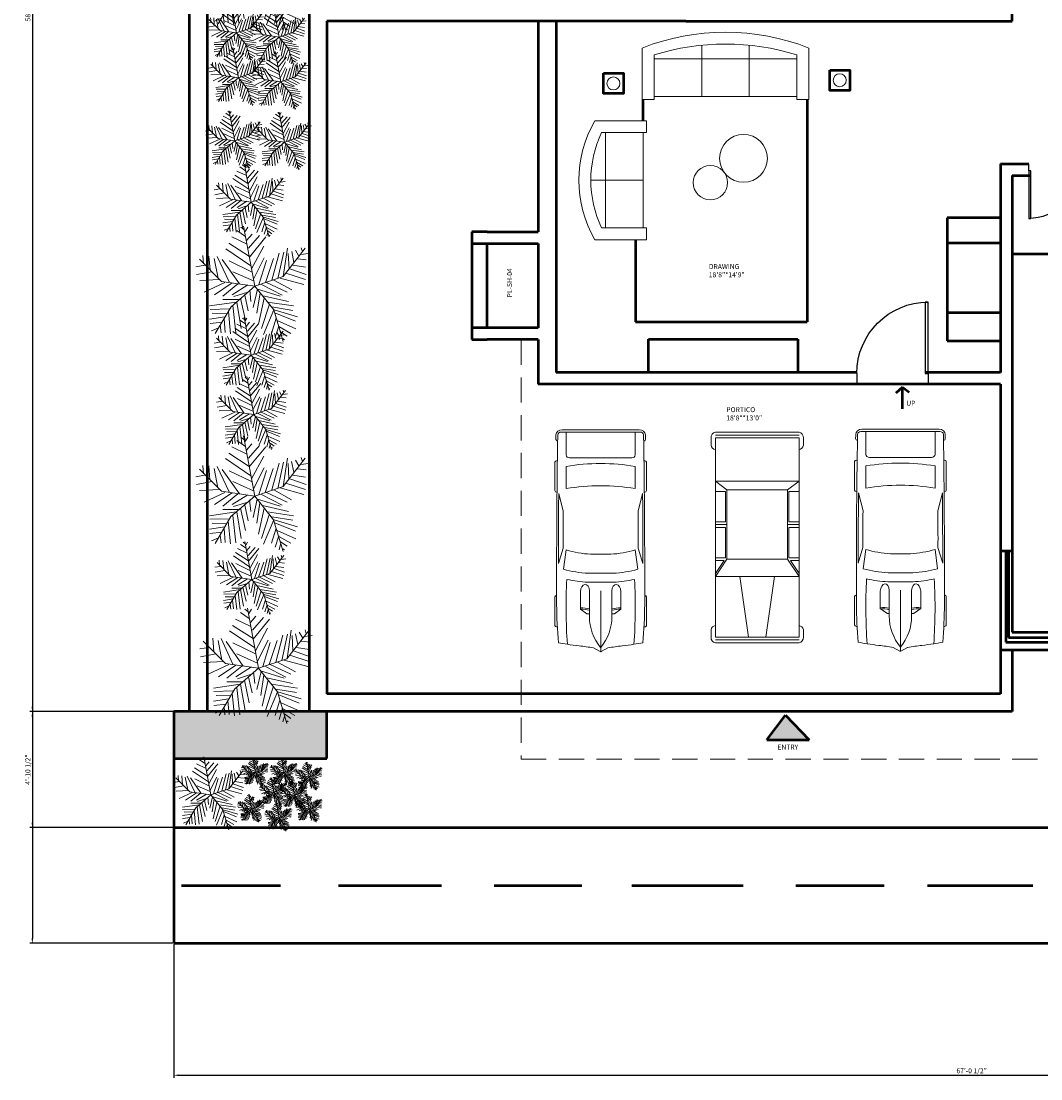
# Model space of a CAD drawing. Units: inches. Extents: x 5312 to 23584, y 2846 to 7447.
# Tile 1 of 12: x 8876 to 9390, y 2846 to 3379. Entities that reach past the tile are written whole.
import ezdxf

# ---------------------------------------------------------------- set-up
doc = ezdxf.new("R2010")
doc.units = ezdxf.units.IN
doc.linetypes.add('DASHED', pattern=[19.05, 12.7, -6.35])
for name, color, linetype, lineweight in [('A-ANNO-DIMS', 2, 'Continuous', 18), ('A-ANNO-TEXT', 3, 'Continuous', 18), ('A-AREA-IDEN', 7, 'Continuous', 18), ('A-DOOR', 4, 'Continuous', 25), ('A-EQPM-VEHI', 8, 'Continuous', 18), ('A-FLOR-OVHD', 8, 'DASHED', 18), ('A-FLOR-PATT', 252, 'Continuous', 13), ('A-FURN', 8, 'Continuous', 18), ('A-WALL', 7, 'Continuous', 50), ('L-PLNT', 82, 'Continuous', 13)]:
    doc.layers.add(name, color=color, linetype=linetype, lineweight=lineweight)
doc.styles.get("Standard").update_dxf_attribs({"font": 'arial.ttf'})
doc.dimstyles.new('ISO-25', dxfattribs={"dimtxt": 2.5, "dimasz": 2.5, "dimexe": 1.25, "dimexo": 0.625, "dimtad": 1, "dimlunit": 3, "dimtxsty": 'Standard', "dimcen": 2.5, "dimadec": 0, "dimazin": 0, "dimtfac": 1, "dimtmove": 0, "dimatfit": 3, "dimfxl": 1, "dimarcsym": 0})

# ---------------------------------------------------------------- blocks, each defined once
blk = doc.blocks.new('Sofa - Roundback 7 ft.')
for p, q in [((-12.00002, -32.4421), (-12.00003, -6.5971)), ((11.99997, -32.4421), (11.99998, -6.5971)), ((-36.000027, -34), (-36.000027, -11.4696)), ((-35.999844, -13.3819), (35.9998, -13.3819)), ((35.99998, -34), (35.99998, -11.4696)), ((-36.000027, -32.4421), (35.99998, -32.4421))]:
    blk.add_line(p, q)
for points in [[(-36.000027, -34), (-42.000027, -34), (-42.000027, -8)], [(41.99998, -8), (41.99998, -34), (35.99998, -34)]]:
    blk.add_lwpolyline(points)
for centre, radius, start, end in [((0, -114.25), 114.25, 68.43141, 111.5686), ((-0.00001, -127.1968), 121.1968, 72.72033, 107.2797)]:
    blk.add_arc(centre, radius, start, end)
blk = doc.blocks.new('Sofa - Roundback Loveseat 5 ft.')
for p, q in [((0, -32.44198), (0, -5.99998)), ((-24, -33.99998), (-24, -11.46958)), ((-23.9998, -13.38178), (23.99986, -13.38178)), ((24.00004, -33.99998), (24.00004, -11.46958)), ((-24, -32.44198), (24.00004, -32.44198))]:
    blk.add_line(p, q)
for points in [[(-24, -33.99998), (-30, -33.99998), (-30, -7.99998)], [(30.00004, -7.99998), (30.00004, -33.99998), (24.00004, -33.99998)]]:
    blk.add_lwpolyline(points)
for centre, radius, start, end in [((0, -60.24998), 60.24998, 60.13715, 119.8628), ((0, -61.38438), 55.38444, 64.32083, 115.6792)]:
    blk.add_arc(centre, radius, start, end)
blk = doc.blocks.new('*U14')
for p, q in [((21.1, 37.41), (21.1, 36.83)), ((46.55, 38.89), (22.35, 38.89)), ((47.8, 37.39), (47.8, 37.41)), ((87.99, 31.87), (74.76, 35.92)), ((135.45, 37.07), (135.45, 37.41)), ((136.7, 38.89), (160.9, 38.89)), ((162.15, 37.41), (162.15, 36.77)), ((70.03, 31.54), (86.41, 29.35)), ((134.31, 35.6), (119.29, 31.78)), ((138.42, 29.35), (157.25, 29.35)), ((186.47, 29.35), (167.01, 29.35)), ((186.47, -33.5), (186.47, 33.5)), ((188.4, -32.76), (188.4, 32.76)), ((164.52, 26.39), (164.52, -26.39)), ((29.77, 9.51), (51.68, 9.51)), ((32.12, 9.51), (32.12, 11.15)), ((32.27, 11.63), (36.13, 17.17)), ((36.13, 17.17), (50.94, 17.17)), ((58.92, -10.77), (58.92, 10.77)), ((66.55, -10.53), (66.55, 10.53)), ((186.47, -10.53), (186.47, 10.53)), ((3.27, 6.13), (0.1, 0.41)), ((82.74, 8.5), (82.74, -8.5)), ((0, 0), (51.68, 0)), ((0.1, -0.41), (3.27, -6.13)), ((29.77, -9.51), (51.68, -9.51)), ((32.12, -9.51), (32.12, -11.15)), ((32.27, -11.63), (36.13, -17.17)), ((36.13, -17.17), (50.94, -17.17)), ((86.41, -29.35), (70.03, -31.54)), ((87.99, -31.87), (74.76, -35.92)), ((134.31, -35.6), (119.29, -31.78)), ((157.25, -29.35), (138.42, -29.35)), ((167.01, -29.35), (186.47, -29.35)), ((21.1, -37.41), (21.1, -36.83)), ((46.55, -38.89), (22.35, -38.89)), ((47.8, -37.39), (47.8, -37.41)), ((135.45, -37.07), (135.45, -37.41)), ((136.7, -38.89), (160.9, -38.89)), ((162.15, -37.41), (162.15, -36.77))]:
    blk.add_line(p, q)
for centre, major_axis, ratio, start_param, end_param in [((41.19, -490.86), (0, 528.23), 0.842304, 0.00281, 0.075598), ((22.35, 37.41), (0, -1.48), 0.842304, 3.141593, 4.712389), ((64.48, -10555.62), (0, 10593.03), 0.842304, -0.013397, 0.002797), ((46.55, 37.41), (0, 1.48), 0.842304, -1.570796, 0), ((64.48, -10555.62), (0, -10591.55), 0.842304, 3.133765, 3.140441), ((136.7, 37.41), (0, -1.48), 0.842304, 3.141593, 4.712389), ((160.9, 37.41), (0, 1.48), 0.842304, -1.570796, 0), ((180.63, 35.84), (0, 2.22), 0.842304, -0.013017, 1.249894), ((64.48, -10556.36), (0, 10595.31), 0.842304, -0.013397, -0.013017), ((183.98, 33.5), (0, -2.96), 0.842304, 1.570796, 3.128196), ((183.98, 32.76), (0, -5.25), 0.842304, 1.570796, 3.128196), ((259.18, -27.52), (0, -305.3), 0.842304, 4.528606, 4.561838), ((266.03, -27.52), (0, 313.31), 0.842304, 1.367076, 1.39176), ((37.47, -593.96), (0, -623.33), 0.842304, 3.096046, 3.200911), ((134.4, 5.39), (0, -89.78), 0.842304, 4.449482, 4.652344), ((135.29, 5.39), (0, 81.77), 0.842304, 1.245306, 1.50788), ((149.6, 2.8), (0, -79.58), 0.842304, 4.372215, 4.640744), ((95.79, -3666.35), (0, -3698.24), 0.842304, 3.134049, 3.144098), ((17.08, 0), (0, 147.02), 0.842304, 4.511394, 4.913384), ((35.91, 0), (0, 147.02), 0.842304, 4.511394, 4.913384), ((167.01, 26.39), (0, 2.96), 0.842304, 0, 1.570796), ((-204.49, 52.4), (0, -250.96), 0.842304, 1.385369, 1.434372), ((29.77, -46.66), (0, 56.17), 0.842304, 0, 0.590319), ((32.75, 11.15), (0, 0.74), 0.842304, 0.879714, 1.570796), ((13.04, 17.01), (0, 27.42), 0.842304, 4.435146, 4.718221), ((14.2, 17.01), (0, 27.42), 0.842304, 4.435146, 4.718221), ((50.79, 13.34), (6.34, -0.36), 0.603834, -1.395552, 1.581315), ((0.62, 0), (0, -0.74), 0.842304, 4.131459, 5.293319), ((-204.49, -52.4), (0, 250.96), 0.842304, -1.434372, -1.385369), ((29.77, 46.66), (0, 56.17), 0.842304, 2.551274, 3.141593), ((149.6, -2.8), (0, -79.58), 0.842304, -1.499151, -1.230623), ((32.75, -11.15), (0, -0.74), 0.842304, 4.712389, 5.403472), ((13.04, -17.01), (0, -27.42), 0.842304, 1.564964, 1.848039), ((14.2, -17.01), (0, -27.42), 0.842304, 1.564964, 1.848039), ((134.4, -5.39), (0, -89.78), 0.842304, -1.510751, -1.307889), ((135.29, -5.39), (0, -81.77), 0.842304, -1.50788, -1.245306), ((259.18, 27.52), (0, 305.3), 0.842304, 1.721348, 1.754579), ((167.01, -26.39), (0, -2.96), 0.842304, 4.712389, 6.283185), ((266.03, 27.52), (0, 313.31), 0.842304, 1.749832, 1.774517), ((37.47, 593.96), (0, -623.33), 0.842304, -0.059319, 0.045547), ((41.19, 490.86), (0, -528.23), 0.842304, -0.075598, -0.00281), ((64.48, 10555.62), (0, -10591.55), 0.842304, 0.001152, 0.007828), ((95.79, 3666.35), (0, -3698.24), 0.842304, -0.002505, 0.007544), ((183.98, -33.5), (0, 2.96), 0.842304, 3.15499, 4.712389), ((183.98, -32.76), (0, -5.25), 0.842304, 0.013397, 1.570796), ((22.35, -37.41), (0, 1.48), 0.842304, 1.570796, 3.141593), ((64.48, 10555.62), (0, 10593.03), 0.842304, 3.138796, 3.15499), ((46.55, -37.41), (0, -1.48), 0.842304, 0, 1.570796), ((136.7, -37.41), (0, -1.48), 0.842304, -1.570796, 0), ((160.9, -37.41), (0, 1.48), 0.842304, 3.141593, 4.712389), ((180.63, -35.84), (0, -2.22), 0.842304, -1.249894, 0.013017), ((64.48, 10556.36), (0, 10595.31), 0.842304, 3.15461, 3.15499)]:
    blk.add_ellipse(centre, major_axis=major_axis, ratio=ratio, start_param=start_param, end_param=end_param)
at = {"extrusion": (0, 0, -1)}
blk.add_ellipse((50.79, -13.34), major_axis=(6.34, 0.36), ratio=0.603834, start_param=-1.395552, end_param=1.581315, dxfattribs=at)
blk = doc.blocks.new('*U15')
for p, q in [((5.44, 42.31), (12.12, 42.31)), ((189.69, 42.31), (183.01, 42.31)), ((0.1, -0.41), (0.1, 38.35)), ((2.77, -0.41), (2.77, 38.31)), ((5.44, -0.41), (5.44, 38.24)), ((5.45, 38.31), (16.12, 38.31)), ((16.12, 38.31), (180.34, 38.31)), ((61.52, -0.41), (61.52, 38.31)), ((61.52, 38.31), (77.54, 27.62)), ((64.19, 38.31), (76.2, 30.29)), ((76.2, 30.29), (76.2, 38.31)), ((78.87, 38.31), (78.87, 28.96)), ((106.91, 28.96), (106.91, 38.31)), ((109.58, 27.62), (109.58, 38.31)), ((112.25, 38.31), (112.25, 28.96)), ((140.29, 28.96), (140.29, 38.31)), ((141.62, 27.62), (149.64, 38.31)), ((149.64, -0.41), (149.64, 38.31)), ((189.69, 38.31), (179.01, 38.31)), ((189.69, -0.41), (189.69, 38.24)), ((192.36, -0.41), (192.36, 38.31)), ((195.03, -0.41), (195.03, 38.35)), ((77.54, 27.62), (141.62, 27.62)), ((77.54, -0.41), (77.54, 27.62)), ((78.87, 28.96), (106.91, 28.96)), ((112.25, 28.96), (140.29, 28.96)), ((141.62, -0.41), (141.62, 27.62)), ((5.44, 7.6), (61.52, 15.61)), ((0.1, -0.42), (0.1, -39.18)), ((2.77, -0.41), (2.77, -39.13)), ((5.44, -0.42), (5.44, -39.07)), ((5.44, -8.42), (61.52, -16.43)), ((61.52, -0.41), (61.52, -39.13)), ((77.54, -0.41), (77.54, -28.45)), ((141.62, -0.41), (141.62, -28.45)), ((149.64, -0.41), (149.64, -39.13)), ((189.69, -0.42), (189.69, -39.07)), ((192.36, -0.41), (192.36, -39.13)), ((195.03, -0.42), (195.03, -39.18)), ((61.52, -39.13), (77.54, -28.45)), ((77.54, -28.45), (141.62, -28.45)), ((109.58, -28.45), (109.58, -39.13)), ((141.62, -28.45), (149.64, -39.13)), ((5.45, -39.13), (16.12, -39.13)), ((16.12, -39.13), (180.34, -39.13)), ((64.19, -39.13), (76.2, -31.12)), ((76.2, -31.12), (76.2, -39.13)), ((78.87, -39.13), (78.87, -29.79)), ((78.87, -29.79), (106.91, -29.79)), ((106.91, -29.79), (106.91, -39.13)), ((112.25, -29.79), (140.29, -29.79)), ((112.25, -39.13), (112.25, -29.79)), ((140.29, -29.79), (140.29, -39.13)), ((189.69, -39.13), (179.01, -39.13)), ((5.44, -43.14), (12.12, -43.14)), ((189.69, -43.14), (183.01, -43.14))]:
    blk.add_line(p, q)
for centre, radius, start, end in [((5.06, 37.26), 5.06, 85.64554, 168.0943), ((11.45, 37.64), 4.72, 8.13011, 81.86996), ((183.68, 37.64), 4.72, 98.13004, 171.8699), ((190.07, 37.26), 5.06, 11.90574, 94.35446), ((5.06, -38.09), 5.06, 191.9057, 274.3545), ((11.45, -38.46), 4.72, 278.13, 351.8699), ((183.68, -38.46), 4.72, 188.1301, 261.87), ((190.07, -38.09), 5.06, 265.6455, 348.0943)]:
    blk.add_arc(centre, radius, start, end)
blk = doc.blocks.new('*U2')
for p, q in [((0, 0), (0, -6)), ((40, 0), (40, -6))]:
    blk.add_line(p, q)
blk.add_lwpolyline([(0, 0), (0, 40), (1.75, 40), (1.75, 0)], close=True)
blk.add_arc((0, 0), 40, 0, 90)
blk = doc.blocks.new('*U18')
for p, q in [((-8.737, 47.138), (-17.069, 52.711)), ((-10.186, 53.64), (-13.084, 55.962)), ((0, 0), (-10.5, 57)), ((-9.099, 51.782), (-6.563, 55.962)), ((-5.114, 28.097), (-24.676, 40.636)), ((-7.288, 39.707), (-21.778, 46.673)), ((-7.65, 43.423), (-2.578, 49.46)), ((-5.839, 35.992), (4.667, 48.067)), ((-5.114, 27.632), (10.463, 46.673)), ((-3.665, 19.273), (-27.574, 35.527)), ((-2.941, 16.486), (8.652, 37.85)), ((16.259, 5.805), (23.142, 31.348)), ((22.055, 7.198), (27.489, 32.277)), ((27, 9), (48, 36)), ((27.127, 9.056), (31.112, 35.992)), ((31.836, 30.883), (32.561, 16.486)), ((35.096, 32.741), (37.27, 22.524)), ((38.719, 34.134), (41.979, 28.561)), ((43.791, 29.954), (51.036, 30.883)), ((44.153, 36.456), (45.239, 32.741)), ((-31.5, 4.5), (-52.5, 25.5)), ((-48.585, 21.131), (-49.309, 29.026)), ((-43.513, 28.561), (-42.427, 15.558)), ((-38.442, 26.239), (-34.819, 7.663)), ((-35.544, 28.097), (-24.314, 3.947)), ((-14.533, 2.09), (-30.834, 25.31)), ((-24.314, 23.917), (-2.941, 13.7)), ((-1.129, 6.734), (9.014, 26.704)), ((3.942, 1.625), (11.187, 24.381)), ((10.101, 3.483), (17.708, 26.239)), ((40.53, 25.775), (48.862, 24.846)), ((-47.498, 19.737), (-55.83, 18.344)), ((-40.615, 13.7), (-55.105, 10.913)), ((-20.691, 13.7), (-1.129, 4.876)), ((29.662, 12.307), (48.137, 6.269)), ((33.285, 16.486), (48.862, 10.913)), ((36.183, 19.737), (48.137, 17.88)), ((-33.37, 6.269), (-52.207, 5.34)), ((-28.299, 3.483), (-47.86, -5.805)), ((-21.416, 3.018), (-38.079, -8.128)), ((0, 0), (-31.5, 4.5)), ((-15.982, 2.09), (-30.11, -9.521)), ((0, 0), (-22.5, -19.5)), ((-6.563, 1.161), (-21.416, -8.128)), ((0, 0), (27, 9)), ((0, 0), (18, -22.5)), ((6.478, 1.625), (26.04, -8.592)), ((11.187, 3.483), (30.749, -5.805)), ((18.07, 5.805), (35.096, -3.483)), ((24.229, 7.663), (46.688, 1.625)), ((-6.563, -5.805), (-19.967, -9.985)), ((-9.461, -8.592), (-6.201, -23.453)), ((-4.752, -3.483), (-3.665, -14.629)), ((2.493, -3.019), (-1.491, -20.202)), ((1.769, -2.555), (24.229, -9.521)), ((5.029, -6.27), (2.131, -25.775)), ((7.565, -9.056), (32.198, -14.629)), ((-17.431, -15.094), (-42.789, -18.809)), ((-22.5, -19.5), (-37.5, -45)), ((-15.257, -12.772), (-30.11, -12.772)), ((-20.691, -18.345), (-17.793, -44.352)), ((-17.069, -15.094), (-12.721, -40.172)), ((-13.446, -11.378), (-8.737, -32.741)), ((9.014, -11.378), (3.58, -35.992)), ((14.085, -16.951), (6.478, -40.172)), ((12.274, -15.094), (36.907, -18.809)), ((16.259, -19.738), (36.183, -22.989)), ((-28.299, -29.026), (-42.789, -31.348)), ((-24.314, -21.596), (-42.427, -22.06)), ((-26.849, -26.24), (-40.253, -25.775)), ((-25.038, -23.918), (-22.865, -45.281)), ((18.07, -22.524), (8.289, -45.745)), ((18, -22.5), (27, -52.5)), ((18.433, -22.524), (40.53, -29.026)), ((19.157, -25.311), (38.719, -33.206)), ((-30.834, -34.135), (-42.427, -35.528)), ((-34.457, -39.708), (-40.978, -42.494)), ((-32.646, -36.921), (-31.921, -44.352)), ((-29.023, -30.884), (-27.936, -43.887)), ((20.244, -30.419), (15.897, -44.816)), ((22.78, -37.85), (19.519, -48.532)), ((21.331, -32.741), (39.081, -40.636)), ((22.78, -38.314), (34.372, -44.816)), ((24.591, -45.745), (23.142, -50.854)), ((24.591, -43.423), (30.749, -47.603)), ((26.764, -49.925), (28.213, -50.854))]:
    blk.add_line(p, q)
blk = doc.blocks.new('*D45')
at = {"layer": 'A-ANNO-DIMS', "color": 0, "lineweight": -2, "transparency": 16777216}
for p, q in [((8952.82, 2913.28), (8952.82, 2846.15)), ((9757.28, 2913.28), (9757.28, 2846.15)), ((8955.32, 2847.4), (9754.78, 2847.4))]:
    blk.add_line(p, q, dxfattribs=at)
at = {"layer": 'A-ANNO-DIMS', "color": 0, "transparency": 16777216}
for points in [[(8955.32, 2847.82), (8955.32, 2846.98), (8952.82, 2847.4)], [(9754.78, 2847.82), (9754.78, 2846.98), (9757.28, 2847.4)]]:
    blk.add_solid(points, dxfattribs=at)
at = {"layer": 'DEFPOINTS', "color": 0, "transparency": 16777216}
for p in [(8952.82, 2913.9), (9757.28, 2913.9), (9757.28, 2847.4)]:
    blk.add_point(p, dxfattribs=at)
at = {"layer": 'A-ANNO-DIMS', "color": 0, "transparency": 16777216, "insert": (9355.05, 2849.32), "char_height": 2.5, "attachment_point": 5}
blk.add_mtext('67\'-0 1/2"', dxfattribs=at)
blk = doc.blocks.new('*D47')
at = {"layer": 'A-ANNO-DIMS', "color": 0, "lineweight": -2, "transparency": 16777216}
for p, q in [((8959.95, 4009.84), (8880.22, 4009.84)), ((8881.47, 4007.34), (8881.47, 2916.4)), ((8952.19, 2913.9), (8880.22, 2913.9))]:
    blk.add_line(p, q, dxfattribs=at)
at = {"layer": 'A-ANNO-DIMS', "color": 0, "transparency": 16777216}
for points in [[(8881.05, 4007.34), (8881.89, 4007.34), (8881.47, 4009.84)], [(8881.05, 2916.4), (8881.89, 2916.4), (8881.47, 2913.9)]]:
    blk.add_solid(points, dxfattribs=at)
at = {"layer": 'DEFPOINTS', "color": 0, "transparency": 16777216}
for p in [(8960.57, 4009.84), (8881.47, 2913.9), (8952.82, 2913.9)]:
    blk.add_point(p, dxfattribs=at)
at = {"layer": 'A-ANNO-DIMS', "color": 0, "transparency": 16777216, "insert": (8879.57, 3461.87), "char_height": 2.5, "attachment_point": 5, "rotation": 90}
blk.add_mtext('91\'-4"', dxfattribs=at)
blk = doc.blocks.new('*D52')
at = {"layer": 'A-ANNO-DIMS', "color": 0, "lineweight": -2, "transparency": 16777216}
for p, q in [((9020.38, 3737.65), (8880.22, 3737.65)), ((8881.47, 3735.15), (8881.47, 3033.15)), ((9020.38, 3030.65), (8880.22, 3030.65))]:
    blk.add_line(p, q, dxfattribs=at)
at = {"layer": 'A-ANNO-DIMS', "color": 0, "transparency": 16777216}
for points in [[(8881.05, 3735.15), (8881.89, 3735.15), (8881.47, 3737.65)], [(8881.05, 3033.15), (8881.89, 3033.15), (8881.47, 3030.65)]]:
    blk.add_solid(points, dxfattribs=at)
at = {"layer": 'DEFPOINTS', "color": 0, "transparency": 16777216}
for p in [(9021.01, 3737.65), (8881.47, 3030.65), (9021.01, 3030.65)]:
    blk.add_point(p, dxfattribs=at)
at = {"layer": 'A-ANNO-DIMS', "color": 0, "transparency": 16777216, "insert": (8879.57, 3384.15), "char_height": 2.5, "attachment_point": 5, "rotation": 90}
blk.add_mtext('58\'-11"', dxfattribs=at)
blk = doc.blocks.new('*D53')
at = {"layer": 'A-ANNO-DIMS', "color": 0, "lineweight": -2, "transparency": 16777216}
for p, q in [((9020.38, 3030.65), (8880.22, 3030.65)), ((8881.47, 3028.15), (8881.47, 2974.77)), ((8952.19, 2972.27), (8880.22, 2972.27))]:
    blk.add_line(p, q, dxfattribs=at)
at = {"layer": 'A-ANNO-DIMS', "color": 0, "transparency": 16777216}
for points in [[(8881.05, 3028.15), (8881.89, 3028.15), (8881.47, 3030.65)], [(8881.05, 2974.77), (8881.89, 2974.77), (8881.47, 2972.27)]]:
    blk.add_solid(points, dxfattribs=at)
at = {"layer": 'DEFPOINTS', "color": 0, "transparency": 16777216}
for p in [(9021.01, 3030.65), (8881.47, 2972.27), (8952.82, 2972.27)]:
    blk.add_point(p, dxfattribs=at)
at = {"layer": 'A-ANNO-DIMS', "color": 0, "transparency": 16777216, "insert": (8879.55, 3001.46), "char_height": 2.5, "attachment_point": 5, "rotation": 90}
blk.add_mtext('4\'-10 1/2"', dxfattribs=at)

msp = doc.modelspace()

# ---------------------------------------------------------------- hatches: boundary and pattern name
at = {"layer": 'A-FLOR-PATT'}
h = msp.add_hatch(dxfattribs=at)
h.set_pattern_fill('ANGLE', color=256)
h.set_pattern_definition([(0, (2182.2664, -374.049), (0, 6.985), [5.08, -1.905]), (90, (2182.2664, -374.049), (-6.985, 4e-16), [5.08, -1.905])])
h.paths.add_polyline_path([(9757.283, 3061.779), (9646.009, 3061.779), (9516.127, 3061.779), (9516.127, 3013.653), (9757.283, 3013.653)])
h.paths.add_polyline_path([(9030.009, 3030.646), (9021.009, 3030.646), (8952.82, 3030.646), (8952.82, 3007.004), (9030.009, 3007.004)])
h = msp.add_hatch(color=256, dxfattribs=at)
h.dxf.hatch_style = 1
h.paths.add_polyline_path([(9261.21, 3028.947), (9251.788, 3016.437), (9273.059, 3016.437)])

# ---------------------------------------------------------------- linework, layer by layer
at = {"layer": 'A-FLOR-OVHD'}
for p, q in [((9127.897, 3218.157), (9127.897, 3006.697)), ((9127.897, 3006.697), (9485.603, 3006.697))]:
    msp.add_line(p, q, dxfattribs=at)
at = {"layer": 'A-FURN'}
for centre, radius in [((9174.444, 3347.259), 3.268), ((9288.548, 3348.879), 3.268), ((9240.037, 3309.499), 12.049), ((9223.372, 3297.248), 8.66)]:
    msp.add_circle(centre, radius, dxfattribs=at)
at = {"layer": 'A-WALL'}
for p, q in [((8960.573, 4009.837), (8960.573, 3030.646)), ((8969.573, 4000.837), (8969.573, 3030.646)), ((9021.009, 3737.646), (9021.009, 3030.646)), ((9375.565, 3378.646), (9375.565, 3384.646)), ((9211.009, 3378.646), (9030.009, 3378.646)), ((9030.009, 3378.646), (9030.009, 3039.646)), ((9136.565, 3378.646), (9136.565, 3272.515)), ((9145.565, 3378.646), (9145.565, 3201.646)), ((9211.009, 3378.646), (9375.565, 3378.646)), ((9189.488, 3328.483), (9189.488, 3339.106)), ((9272.158, 3339.106), (9272.158, 3227.095)), ((9369.565, 3306.779), (9369.565, 3201.646)), ((9369.565, 3306.779), (9383.833, 3306.779)), ((9375.565, 3300.779), (9375.565, 3070.779)), ((9375.565, 3300.779), (9384.883, 3300.779)), ((9369.565, 3279.601), (9342.694, 3279.601)), ((9342.694, 3279.601), (9342.694, 3217.574)), ((9110.742, 3272.515), (9103.059, 3272.515)), ((9103.059, 3272.515), (9103.059, 3218.157)), ((9110.742, 3272.515), (9136.565, 3272.515)), ((9185.632, 3268.483), (9185.632, 3227.095)), ((9103.059, 3266.515), (9136.565, 3266.515)), ((9110.742, 3224.157), (9110.742, 3266.515)), ((9136.565, 3266.515), (9136.565, 3224.157)), ((9342.694, 3266.938), (9369.565, 3266.938)), ((9375.565, 3261.354), (9413.869, 3261.354)), ((9342.694, 3231.84), (9369.565, 3231.84)), ((9185.632, 3227.095), (9272.158, 3227.095)), ((9136.565, 3224.157), (9103.059, 3224.157)), ((9103.059, 3218.157), (9110.742, 3218.157)), ((9136.565, 3218.157), (9110.742, 3218.157)), ((9136.565, 3218.157), (9136.565, 3195.646)), ((9192.11, 3201.646), (9192.11, 3218.332)), ((9192.11, 3218.332), (9267.407, 3218.332)), ((9267.407, 3218.332), (9267.407, 3201.646)), ((9342.694, 3217.574), (9369.565, 3217.574)), ((9297.124, 3201.646), (9145.565, 3201.646)), ((9369.565, 3201.646), (9331.544, 3201.646)), ((9369.565, 3195.646), (9136.565, 3195.646)), ((9320.115, 3194.131), (9316.769, 3191.204)), ((9320.115, 3183.267), (9320.115, 3194.131)), ((9320.115, 3194.131), (9323.483, 3191.662)), ((9369.565, 3195.646), (9369.565, 3039.646)), ((9369.565, 3111.733), (9375.565, 3111.733)), ((9372.219, 3111.708), (9372.219, 3065.688)), ((9373.71, 3111.733), (9373.71, 3068.089)), ((9375.565, 3070.779), (9563.009, 3070.779)), ((9372.219, 3065.688), (9431.962, 3065.688)), ((9373.71, 3068.089), (9431.962, 3068.089)), ((9369.565, 3061.779), (9646.009, 3061.779)), ((9375.565, 3061.779), (9375.565, 3030.646)), ((9369.565, 3039.646), (9030.009, 3039.646)), ((9021.009, 3030.646), (8952.82, 3030.646)), ((8952.82, 3030.646), (8952.82, 2913.9)), ((9375.565, 3030.646), (9021.009, 3030.646)), ((9030.009, 3007.004), (9030.009, 3030.646)), ((9251.788, 3016.437), (9261.21, 3028.947)), ((9261.21, 3028.947), (9273.059, 3016.437)), ((9251.788, 3016.437), (9273.059, 3016.437)), ((8952.82, 3007.004), (9030.009, 3007.004)), ((8952.82, 2972.273), (9757.283, 2972.273)), ((8956.627, 2943.087), (9006.566, 2943.087)), ((9035.887, 2943.087), (9087.733, 2943.087)), ((9114.369, 2943.087), (9158.593, 2943.087)), ((9183.688, 2943.087), (9239.834, 2943.087)), ((9266.434, 2943.087), (9310.873, 2943.087)), ((9332.863, 2943.087), (9385.967, 2943.087)), ((8952.82, 2913.9), (9757.283, 2913.9))]:
    msp.add_line(p, q, dxfattribs=at)
for points in [[(9283.528, 3354.017), (9293.568, 3354.017), (9293.568, 3343.741), (9283.528, 3343.741)], [(9169.424, 3352.397), (9179.464, 3352.397), (9179.464, 3342.121), (9169.424, 3342.121)]]:
    msp.add_lwpolyline(points, close=True, dxfattribs=at)

# ---------------------------------------------------------------- block references
at = {"layer": 'A-DOOR', "xscale": -0.6, "yscale": 0.6, "zscale": 0.6, "rotation": 180}
msp.add_blockref('*U2', (9383.833, 3303.179), dxfattribs=at)
at = {"layer": 'A-DOOR', "xscale": -0.9, "yscale": 0.9, "zscale": 0.9}
msp.add_blockref('*U2', (9333.119, 3201.046), dxfattribs=at)
at = {"layer": 'A-EQPM-VEHI', "rotation": 90}
for name, p, xscale, yscale, zscale in [('*U14', (9168.017, 3060.861), 0.5937383899157203, 0.5937383899157203, 0.5937383899157203), ('*U14', (9319.163, 3061.107), 0.5937383899157203, 0.5937383899157203, 0.5937383899157203), ('*U15', (9246.738, 3065.264), 0.5446154687930189, 0.5446154687930189, 0.5446154687930189)]:
    msp.add_blockref(name, p, dxfattribs=dict(at, xscale=xscale, yscale=yscale, zscale=zscale))
at = {"layer": 'A-FURN'}
msp.add_blockref('Sofa - Roundback 7 ft.', (9230.952, 3373.106), dxfattribs=at)
at = {"layer": 'A-FURN', "rotation": 89.99999999999999}
msp.add_blockref('Sofa - Roundback Loveseat 5 ft.', (9157.046, 3298.483), dxfattribs=at)
at = {"layer": 'L-PLNT'}
for p, xscale, yscale, zscale in [((8995.071, 3401.266), 0.5312656759052281, 0.5312656759052281, 0.5312656759052281), ((8984.482, 3372.686), 0.2657412829208717, 0.2657412829208717, 0.2657412829208717), ((9005.902, 3370.648), 0.2657412829208717, 0.2657412829208717, 0.2657412829208717), ((8985.349, 3350.159), 0.2657412829208717, 0.2657412829208717, 0.2657412829208717), ((9006.769, 3348.121), 0.2657412829208717, 0.2657412829208717, 0.2657412829208717), ((8983.532, 3318.277), 0.2657412829208717, 0.2657412829208717, 0.2657412829208717), ((9008.645, 3317.709), 0.2657412829208717, 0.2657412829208717, 0.2657412829208717), ((8991.88, 3287.477), 0.3351400291328743, 0.3351400291328743, 0.3351400291328743), ((8993.595, 3245.099), 0.5312656759052281, 0.5312656759052281, 0.5312656759052281), ((8991.838, 3210.285), 0.3351400291328743, 0.3351400291328743, 0.3351400291328743), ((8993.085, 3180.435), 0.3351400291328743, 0.3351400291328743, 0.3351400291328743), ((8993.567, 3139.295), 0.5312656759052281, 0.5312656759052281, 0.5312656759052281), ((8992.174, 3097.236), 0.3351400291328743, 0.3351400291328743, 0.3351400291328743), ((8995.515, 3052.543), 0.5312656759052281, 0.5312656759052281, 0.5312656759052281), ((8971.479, 2988.755), 0.3351400291328743, 0.3351400291328743, 0.3351400291328743), ((8993.943, 2999.916), 0.1284293448203393, 0.1284293448203393, 0.1284293448203393), ((9008.45, 2999.916), 0.1284293448203393, 0.1284293448203393, 0.1284293448203393), ((9021.024, 2997.79), 0.1284293448203393, 0.1284293448203393, 0.1284293448203393), ((9003.159, 2990.034), 0.1284293448203393, 0.1284293448203393, 0.1284293448203393), ((9013.576, 2988.61), 0.1284293448203393, 0.1284293448203393, 0.1284293448203393), ((8992.008, 2981.623), 0.1284293448203393, 0.1284293448203393, 0.1284293448203393), ((9021.024, 2981.748), 0.1284293448203393, 0.1284293448203393, 0.1284293448203393), ((9005.839, 2977.206), 0.1284293448203393, 0.1284293448203393, 0.1284293448203393)]:
    msp.add_blockref('*U18', p, dxfattribs=dict(at, xscale=xscale, yscale=yscale, zscale=zscale))

# ---------------------------------------------------------------- texts
at = {"layer": 'A-ANNO-TEXT', "insert": (9120.835, 3239.413), "char_height": 2.5, "attachment_point": 1, "rotation": 90}
msp.add_mtext_dynamic_manual_height_columns('PL-SH-04', width=15.83459, gutter_width=12.5, heights=[0], dxfattribs=at)
at = {"layer": 'A-ANNO-TEXT', "char_height": 2.5, "attachment_point": 1}
for s, width, insert in [('UP', 6.72881, (9322.121, 3187.349)), ('ENTRY', 19.33564, (9257.136, 3014.048))]:
    msp.add_mtext_dynamic_manual_height_columns(s, width=width, gutter_width=12.5, heights=[0], dxfattribs=dict(at, insert=insert))
at = {"layer": 'A-AREA-IDEN', "char_height": 2.5, "attachment_point": 1}
for s, width, insert in [('DRAWING\\P18\'8"*14\'9"', 49.26695, (9222.548, 3256.225)), ('PORTICO\\P18\'8"*13\'0"', 35.93223, (9231.35, 3184.094))]:
    msp.add_mtext_dynamic_manual_height_columns(s, width=width, gutter_width=12.5, heights=[0], dxfattribs=dict(at, insert=insert))

# ---------------------------------------------------------------- dimensions: what is measured, and where the dimension line sits
at = {"layer": 'A-ANNO-DIMS'}
for base, p1, p2, picture, middle in [((8881.47, 2913.9), (8960.573, 4009.837), (8952.82, 2913.9), '*D47', (8879.569, 3461.869)), ((8881.47, 3030.646), (9021.009, 3737.646), (9021.009, 3030.646), '*D52', (8879.569, 3384.146)), ((8881.47, 2972.273), (9021.009, 3030.646), (8952.82, 2972.273), '*D53', (8879.553, 3001.46))]:
    dim = msp.add_linear_dim(base=base, p1=p1, p2=p2, angle=90, dimstyle='ISO-25', override={"dimdec": 1, "dimlfac": 1, "dimrnd": 0, "dimzin": 1, "dimdsep": 46, "dimlunit": 4, "dimfrac": 2}, dxfattribs=at)
    dim.commit()
    dim.dimension.update_dxf_attribs({"geometry": picture, "text_midpoint": middle})
dim = msp.add_linear_dim(base=(9757.283, 2847.4), p1=(8952.82, 2913.9), p2=(9757.283, 2913.9), dimstyle='ISO-25', override={"dimdec": 1, "dimlfac": 1, "dimrnd": 0, "dimzin": 1, "dimdsep": 46, "dimlunit": 4, "dimfrac": 2}, dxfattribs=at)
dim.commit()
dim.dimension.update_dxf_attribs({"geometry": '*D45', "text_midpoint": (9355.051, 2849.318)})

doc.saveas('drawing.dxf')
